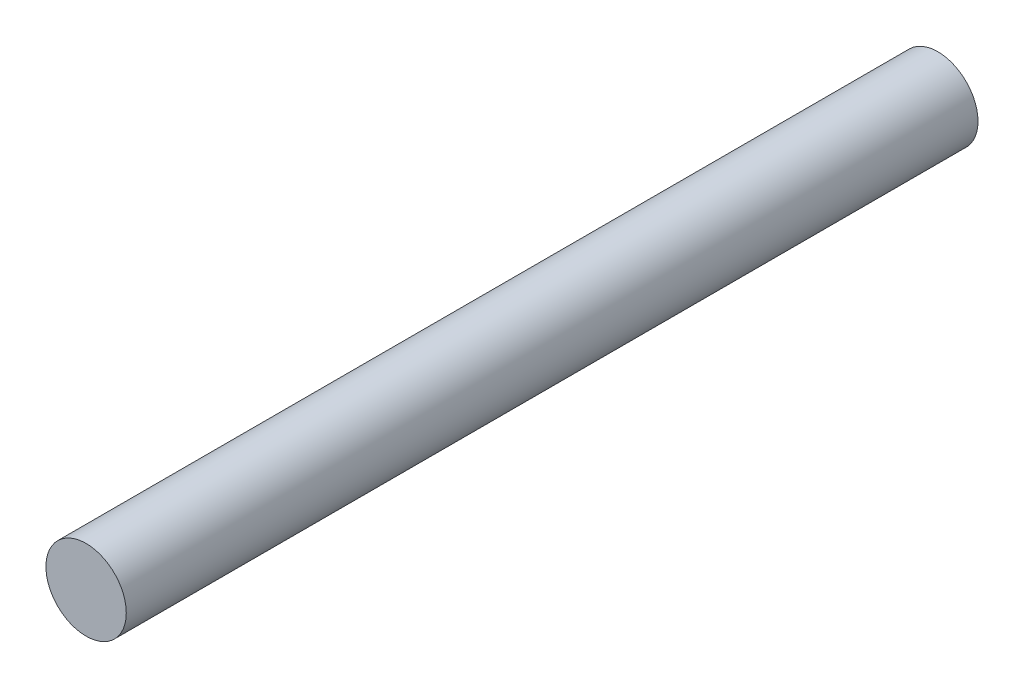
from build123d import *

# Parameters (mm, degrees)
ROD_PROFILE_5_R    = 2.5
ROD_BODY_L53_DEPTH = 26.5


with BuildPart() as part:
    # Rod Profile Ø5 → Rod Body L53 (new, symmetric)
    with BuildSketch(Plane.XY):
        Circle(ROD_PROFILE_5_R)
    extrude(amount=ROD_BODY_L53_DEPTH, both=True)


solid = part.part
